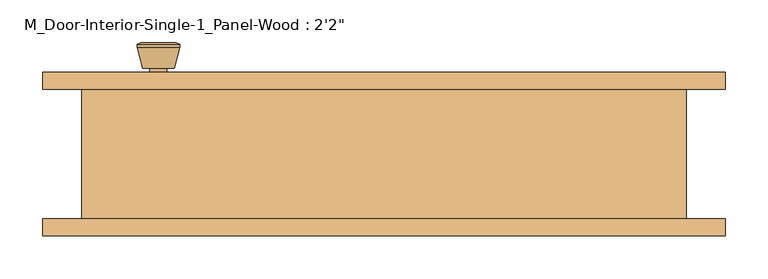
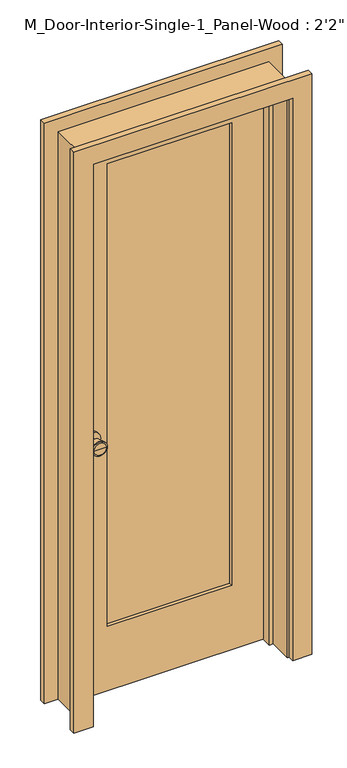
"""IFC4 building model written with IfcOpenShell, lengths in millimetres: door geometry."""

from ifc_helpers import new_model, si_unit, point, frame, frame_2d, origin, place, context, project, spatial, polyline, circle_curve, trimmed, segment, composite_curve, outline, extrude, faceted_brep, source, transform, mapped, element, save
from ifc_brep_helpers import plane_surface, cylinder_surface, revolved_surface, advanced_brep


def door_69f71937(model_context):
    return source(origin(), model_context, "Body", "SolidModel", [
        advanced_brep(
        [(-265.2, 32.025, 914.4), (-255.2, 32.025, 914.4), (-275.2, 32.025, 914.4), (-244.7241324, -16.975, 914.4), (-265.2, -16.975, 914.4), (-285.6758676, -16.975, 914.4), (-240.2, -15.1471319, 914.4), (-290.2, -15.1471319, 914.4), (-240.2, -11.6834537, 914.4), (-290.2, -11.6834537, 914.4), (-246.563764, 13.025, 914.4), (-283.836236, 13.025, 914.4), (-255.2, 13.025, 914.4), (-275.2, 13.025, 914.4)],
        [
            (0, 1),
            (1, 2, circle_curve(frame((-265.2, 32.025, 914.4), z_axis=(0.0, 1.0, 0.0), x_axis=(-1.0, 0.0, 0.0)), 10.0)),
            (2, 0),
            (2, 1, circle_curve(frame((-265.2, 32.025, 914.4), z_axis=(0.0, 1.0, 0.0), x_axis=(-1.0, 0.0, 0.0)), 10.0)),
            (3, 4),
            (4, 5),
            (5, 3, circle_curve(frame((-265.2, -16.975, 914.4), z_axis=(0.0, -1.0, 0.0), x_axis=(-1.0, 0.0, 0.0)), 20.4758676)),
            (3, 5, circle_curve(frame((-265.2, -16.975, 914.4), z_axis=(0.0, -1.0, 0.0), x_axis=(-1.0, 0.0, 0.0)), 20.4758676)),
            (6, 3),
            (5, 7),
            (7, 6, circle_curve(frame((-265.2, -15.1471319, 914.4), z_axis=(0.0, -1.0, 0.0), x_axis=(-1.0, 0.0, 0.0)), 25.0)),
            (6, 7, circle_curve(frame((-265.2, -15.1471319, 914.4), z_axis=(0.0, -1.0, 0.0), x_axis=(-1.0, 0.0, 0.0)), 25.0)),
            (8, 6),
            (7, 9),
            (9, 8, circle_curve(frame((-265.2, -11.6834537, 914.4), z_axis=(0.0, -1.0, 0.0), x_axis=(-1.0, 0.0, 0.0)), 25.0)),
            (8, 9, circle_curve(frame((-265.2, -11.6834537, 914.4), z_axis=(0.0, -1.0, 0.0), x_axis=(-1.0, 0.0, 0.0)), 25.0)),
            (10, 8),
            (9, 11),
            (11, 10, circle_curve(frame((-265.2, 13.025, 914.4), z_axis=(0.0, -1.0, 0.0), x_axis=(-1.0, 0.0, 0.0)), 18.636236)),
            (10, 11, circle_curve(frame((-265.2, 13.025, 914.4), z_axis=(0.0, -1.0, 0.0), x_axis=(-1.0, 0.0, 0.0)), 18.636236)),
            (12, 10),
            (11, 13),
            (13, 12, circle_curve(frame((-265.2, 13.025, 914.4), z_axis=(0.0, -1.0, 0.0), x_axis=(-1.0, 0.0, 0.0)), 10.0)),
            (12, 13, circle_curve(frame((-265.2, 13.025, 914.4), z_axis=(0.0, -1.0, 0.0), x_axis=(-1.0, 0.0, 0.0)), 10.0)),
            (1, 12),
            (13, 2),
        ],
        [
            plane_surface(frame((-265.2, 32.025, 914.4), z_axis=(0.0, 1.0, 0.0), x_axis=(-1.0, 0.0, 0.0))),
            plane_surface(frame((-265.2, -16.975, 914.4), z_axis=(0.0, -1.0, 0.0), x_axis=(-1.0, 0.0, 0.0))),
            revolved_surface(polyline([(-285.6758676, -16.975, 914.4), (-290.2, -15.1471319, 914.4)]), (-265.2, 32.025, 914.4), (0.0, 1.0, 0.0)),
            cylinder_surface(frame((-265.2, 32.025, 914.4), z_axis=(0.0, 1.0, 0.0), x_axis=(-1.0, 0.0, 0.0)), 25.0),
            revolved_surface(polyline([(-290.2, -11.6834537, 914.4), (-283.836236, 13.025, 914.4)]), (-265.2, 32.025, 914.4), (0.0, 1.0, 0.0)),
            plane_surface(frame((-265.2, 13.025, 914.4), z_axis=(0.0, 1.0, 0.0), x_axis=(-1.0, 0.0, 0.0))),
            cylinder_surface(frame((-265.2, 32.025, 914.4), z_axis=(0.0, 1.0, 0.0), x_axis=(-1.0, 0.0, 0.0)), 10.0),
        ],
        [
            (0, [[1, 2, 3]]),
            (0, [[-3, 4, -1]]),
            (1, [[5, 6, 7]]),
            (1, [[-6, -5, 8]]),
            (2, [[9, -7, 10, 11]]),
            (2, [[-10, -8, -9, 12]]),
            (3, [[13, -11, 14, 15]]),
            (3, [[-14, -12, -13, 16]]),
            (4, [[17, -15, 18, 19]]),
            (4, [[-18, -16, -17, 20]]),
            (5, [[21, -19, 22, 23]]),
            (5, [[-22, -20, -21, 24]]),
            (6, [[25, -23, 26, -2]]),
            (6, [[-26, -24, -25, -4]]),
        ],
    ),
        extrude(outline(composite_curve([segment(trimmed(circle_curve(frame_2d((914.4, -265.2)), 30.0), [point((914.4, -295.2))], [point((914.4, -235.2))], False, "CARTESIAN"), True, "CONTINUOUS"), segment(trimmed(circle_curve(frame_2d((914.4, -265.2)), 30.0), [point((914.4, -235.2))], [point((914.4, -295.2))], False, "CARTESIAN"), True, "CONTINUOUS")], self_intersect=False)), frame((0.0, 32.025, 0.0), z_axis=(0.0, 1.0, 0.0), x_axis=(0.0, 0.0, 1.0)), (0.0, 0.0, 1.0), 6.0),
        advanced_brep(
        [(-265.2, 79.025, 914.4), (-275.2, 79.025, 914.4), (-255.2, 79.025, 914.4), (-244.7241324, 128.025, 914.4), (-285.6758676, 128.025, 914.4), (-265.2, 128.025, 914.4), (-240.2, 126.1971319, 914.4), (-290.2, 126.1971319, 914.4), (-240.2, 122.7334537, 914.4), (-290.2, 122.7334537, 914.4), (-246.563764, 98.025, 914.4), (-283.836236, 98.025, 914.4), (-255.2, 98.025, 914.4), (-275.2, 98.025, 914.4)],
        [
            (0, 1),
            (1, 2, circle_curve(frame((-265.2, 79.025, 914.4), z_axis=(0.0, -1.0, 0.0), x_axis=(-1.0, 0.0, 0.0)), 10.0)),
            (2, 0),
            (2, 1, circle_curve(frame((-265.2, 79.025, 914.4), z_axis=(0.0, -1.0, 0.0), x_axis=(-1.0, 0.0, 0.0)), 10.0)),
            (3, 4, circle_curve(frame((-265.2, 128.025, 914.4), z_axis=(0.0, 1.0, 0.0), x_axis=(-1.0, 0.0, 0.0)), 20.4758676)),
            (4, 5),
            (5, 3),
            (4, 3, circle_curve(frame((-265.2, 128.025, 914.4), z_axis=(0.0, 1.0, 0.0), x_axis=(-1.0, 0.0, 0.0)), 20.4758676)),
            (6, 7, circle_curve(frame((-265.2, 126.1971319, 914.4), z_axis=(0.0, 1.0, 0.0), x_axis=(-1.0, 0.0, 0.0)), 25.0)),
            (7, 4),
            (3, 6),
            (7, 6, circle_curve(frame((-265.2, 126.1971319, 914.4), z_axis=(0.0, 1.0, 0.0), x_axis=(-1.0, 0.0, 0.0)), 25.0)),
            (8, 9, circle_curve(frame((-265.2, 122.7334537, 914.4), z_axis=(0.0, 1.0, 0.0), x_axis=(-1.0, 0.0, 0.0)), 25.0)),
            (9, 7),
            (6, 8),
            (9, 8, circle_curve(frame((-265.2, 122.7334537, 914.4), z_axis=(0.0, 1.0, 0.0), x_axis=(-1.0, 0.0, 0.0)), 25.0)),
            (10, 11, circle_curve(frame((-265.2, 98.025, 914.4), z_axis=(0.0, 1.0, 0.0), x_axis=(-1.0, 0.0, 0.0)), 18.636236)),
            (11, 9),
            (8, 10),
            (11, 10, circle_curve(frame((-265.2, 98.025, 914.4), z_axis=(0.0, 1.0, 0.0), x_axis=(-1.0, 0.0, 0.0)), 18.636236)),
            (12, 13, circle_curve(frame((-265.2, 98.025, 914.4), z_axis=(0.0, 1.0, 0.0), x_axis=(-1.0, 0.0, 0.0)), 10.0)),
            (13, 11),
            (10, 12),
            (13, 12, circle_curve(frame((-265.2, 98.025, 914.4), z_axis=(0.0, 1.0, 0.0), x_axis=(-1.0, 0.0, 0.0)), 10.0)),
            (1, 13),
            (12, 2),
        ],
        [
            plane_surface(frame((-265.2, 79.025, 914.4), z_axis=(0.0, -1.0, 0.0), x_axis=(-1.0, 0.0, 0.0))),
            plane_surface(frame((-265.2, 128.025, 914.4), z_axis=(0.0, 1.0, 0.0), x_axis=(-1.0, 0.0, 0.0))),
            revolved_surface(polyline([(-285.6758676, 128.025, 914.4), (-290.2, 126.1971319, 914.4)]), (-265.2, 79.025, 914.4), (0.0, -1.0, 0.0)),
            cylinder_surface(frame((-265.2, 79.025, 914.4), z_axis=(0.0, -1.0, 0.0), x_axis=(-1.0, 0.0, 0.0)), 25.0),
            revolved_surface(polyline([(-290.2, 122.7334537, 914.4), (-283.836236, 98.025, 914.4)]), (-265.2, 79.025, 914.4), (0.0, -1.0, 0.0)),
            plane_surface(frame((-265.2, 98.025, 914.4), z_axis=(0.0, -1.0, 0.0), x_axis=(-1.0, 0.0, 0.0))),
            cylinder_surface(frame((-265.2, 79.025, 914.4), z_axis=(0.0, -1.0, 0.0), x_axis=(-1.0, 0.0, 0.0)), 10.0),
        ],
        [
            (0, [[1, 2, 3]]),
            (0, [[-3, 4, -1]]),
            (1, [[5, 6, 7]]),
            (1, [[8, -7, -6]]),
            (2, [[9, 10, -5, 11]]),
            (2, [[12, -11, -8, -10]]),
            (3, [[13, 14, -9, 15]]),
            (3, [[16, -15, -12, -14]]),
            (4, [[17, 18, -13, 19]]),
            (4, [[20, -19, -16, -18]]),
            (5, [[21, 22, -17, 23]]),
            (5, [[24, -23, -20, -22]]),
            (6, [[-2, 25, -21, 26]]),
            (6, [[-4, -26, -24, -25]]),
        ],
    ),
        extrude(outline(composite_curve([segment(trimmed(circle_curve(frame_2d((914.4, -265.2)), 30.0), [point((914.4, -295.2))], [point((914.4, -235.2))], False, "CARTESIAN"), True, "CONTINUOUS"), segment(trimmed(circle_curve(frame_2d((914.4, -265.2)), 30.0), [point((914.4, -235.2))], [point((914.4, -295.2))], False, "CARTESIAN"), True, "CONTINUOUS")], self_intersect=False)), frame((0.0, 73.025, 0.0), z_axis=(0.0, 1.0, 0.0), x_axis=(0.0, 0.0, 1.0)), (0.0, 0.0, 1.0), 6.0),
        faceted_brep([(355.2, 73.025, 0.0), (355.2, -79.375, 0.0), (330.2, -79.375, 0.0), (330.2, 3.1, 0.0), (317.5, 3.1, 0.0), (317.5, 38.025, 0.0), (330.2, 38.025, 0.0), (330.2, 73.025, 0.0), (355.2, 73.025, 2025.0), (355.2, -79.375, 2025.0), (-355.2, -79.375, 2025.0), (-355.2, -79.375, 0.0), (-330.2, -79.375, 0.0), (-330.2, -79.375, 2000.0), (330.2, -79.375, 2000.0), (330.2, 3.1, 2000.0), (-330.2, 3.1, 2000.0), (-330.2, 3.1, 0.0), (-317.5, 3.1, 0.0), (-317.5, 3.1, 1987.3), (317.5, 3.1, 1987.3), (317.5, 38.025, 1987.3), (-317.5, 38.025, 1987.3), (-317.5, 38.025, 0.0), (-330.2, 38.025, 0.0), (-330.2, 38.025, 2000.0), (330.2, 38.025, 2000.0), (330.2, 73.025, 2000.0), (-330.2, 73.025, 2000.0), (-330.2, 73.025, 0.0), (-355.2, 73.025, 0.0), (-355.2, 73.025, 2025.0)], [[[0, 1, 2, 3, 4, 5, 6, 7]], [[1, 0, 8, 9]], [[2, 1, 9, 10, 11, 12, 13, 14]], [[3, 2, 14, 15]], [[4, 3, 15, 16, 17, 18, 19, 20]], [[5, 4, 20, 21]], [[6, 5, 21, 22, 23, 24, 25, 26]], [[7, 6, 26, 27]], [[0, 7, 27, 28, 29, 30, 31, 8]], [[9, 8, 31, 10]], [[15, 14, 13, 16]], [[21, 20, 19, 22]], [[27, 26, 25, 28]], [[30, 29, 24, 23, 18, 17, 12, 11]], [[10, 31, 30, 11]], [[16, 13, 12, 17]], [[22, 19, 18, 23]], [[28, 25, 24, 29]]]),
        extrude(outline(polyline([(2000.0, -330.2), (0.0, -330.2), (0.0, 330.2), (2000.0, 330.2), (2000.0, -330.2)]), holes=[polyline([(1880.0, -210.2), (1880.0, 210.2), (230.0, 210.2), (230.0, -210.2), (1880.0, -210.2)])]), frame((0.0, 38.025, 0.0), z_axis=(0.0, 1.0, 0.0), x_axis=(0.0, 0.0, 1.0)), (0.0, 0.0, 1.0), 35.0),
        extrude(outline(polyline([(210.2, 49.6916667), (-210.2, 49.6916667), (-210.2, 61.3583333), (210.2, 61.3583333), (210.2, 49.6916667)])), frame((0.0, 0.0, 230.0), z_axis=(0.0, 0.0, 1.0), x_axis=(1.0, 0.0, 0.0)), (0.0, 0.0, 1.0), 1650.0),
        extrude(outline(polyline([(0.0, 336.55), (0.0, 401.55), (2071.35, 401.55), (2071.35, -401.55), (0.0, -401.55), (0.0, -336.55), (2006.35, -336.55), (2006.35, 336.55), (0.0, 336.55)])), frame((0.0, 73.025, 0.0), z_axis=(0.0, 1.0, 0.0), x_axis=(0.0, 0.0, 1.0)), (0.0, 0.0, 1.0), 20.0),
        extrude(outline(polyline([(0.0, 336.55), (0.0, 401.55), (2071.35, 401.55), (2071.35, -401.55), (0.0, -401.55), (0.0, -336.55), (2006.35, -336.55), (2006.35, 336.55), (0.0, 336.55)])), frame((0.0, -99.375, 0.0), z_axis=(0.0, 1.0, 0.0), x_axis=(0.0, 0.0, 1.0)), (0.0, 0.0, 1.0), 20.0),
    ])


if __name__ == "__main__":
    model = new_model("IFC4")
    model_context = context("Model", 3, world=origin())
    ifc_project = project(units=[si_unit("LENGTHUNIT", "METRE", prefix="MILLI")], contexts=[model_context])
    site = spatial("IfcSite", under=ifc_project)
    building = spatial("IfcBuilding", under=site)
    placement = place(None, origin())
    door_shape = door_69f71937(model_context)
    element("IfcDoor", 1, ObjectType="M_Door-Interior-Single-1_Panel-Wood : 2'2\"", at=placement, inside=building, context=model_context, shape_type="MappedRepresentation", body=[
        mapped(door_shape, transform((0.0, 0.0, 0.0), x_axis=(1.0, 0.0, 0.0), y_axis=(0.0, 1.0, 0.0), z_axis=(0.0, 0.0, 1.0))),
    ])
    save(model, "model.ifc")

# Revit data of these elements
# Type "M_Door-Interior-Single-1_Panel-Wood : 2'2\""
#   Type Mark = "17"
#   Assembly Code = "C1020300"
#   Analytic Construction = "Wooden"
#   Top Rail = 0' - 4.72441"
#   Thickness = 0' - 1.37795"
#   Thermal Resistance (R) = 2.5876 (h·ft²·°F)/BTU
#   Swing Angle [instance default] = 90.00°
#   Stiles = 0' - 4.72441"
#   Rough Width = 2' - 3.9685"
#   Rough Height = 6' - 7.72441"
#   Height = 6' - 6.74016"
#   Width = 2' - 2"
#   Heat Transfer Coefficient (U) = 0.3865 BTU/(h·ft²·°F)
#   Bottom Rail = 0' - 9.05512"
#   Trim Material = Cherry
#   Panel Material = Cherry
#   Frame Material = Cherry
#   Door Handle Material = Aluminum
#   Visual Light Transmittance = 0
#   Solar Heat Gain Coefficient = 0
#   Wall Closure = (empty or 0)
#   Function = (empty or 0)
# Element 1 (IfcDoor, "M_Door-Interior-Single-1_Panel-Wood : 2'2\"")
#   Materials on its faces: "Cherry", "Aluminum"
# Materials
#   "Cherry": class "Wood", colour RGB 226 177 128, transparency 0, Description = "Prunus Serotina", Cost = 0
#   "Aluminum": class "Metal", colour RGB 247 247 247, transparency 0, Description = "Aluminum 6061", Cost = 0
